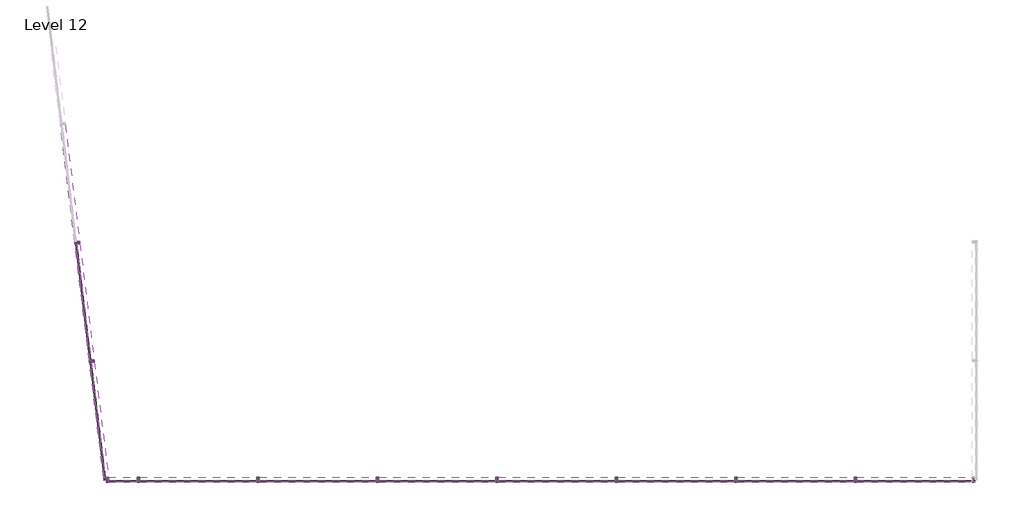
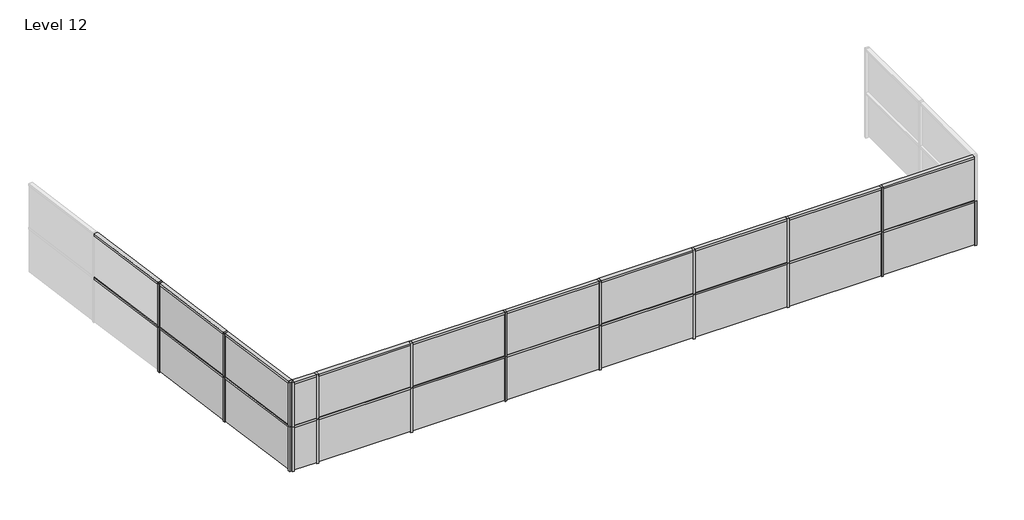
# One storey, part 1 of 2: 45 members, 20 plates.
"""IFC4 building model written with IfcOpenShell, lengths in millimetres."""

from ifc_helpers import new_model, si_unit, origin, place, context, project, spatial, transform, mapped, element, save
from components import member_daa7a266, member_82905deb, member_19d0a4ec, member_8cef0660, member_db480205, member_4491d118, member_0c11e56c, member_695b83e4, system_panel_glazed_37f15d2e, system_panel_glazed_3620f98e, system_panel_glazed_e46d4b42, system_panel_glazed_2a6c68b7, system_panel_glazed_07b088f8, system_panel_glazed_9d0e0944

model = new_model("IFC4")

# Units and contexts
model_context = context("Model", 3, world=origin())
ifc_project = project(units=[si_unit("LENGTHUNIT", "METRE", prefix="MILLI")], contexts=[model_context])

# Site, building, storey
site = spatial("IfcSite", under=ifc_project)
building = spatial("IfcBuilding", under=site)
storey = spatial("IfcBuildingStorey", under=building, Name="Level 12", Elevation=33528.0)

# Members
placement = place(None, origin())
member_shape = member_daa7a266(model_context)
element("IfcMember", 1, ObjectType="Rectangular Mullion : 2.5\" x 5\" rectangular", at=placement, inside=storey, context=model_context, shape_type="MappedRepresentation", body=[
    mapped(member_shape, transform((-8260.4765148, -6916.1096898, 36576.0), x_axis=(0.0, 0.0, 1.0), y_axis=(-0.9925461516413222, -0.12186934340514587, 0.0), z_axis=(0.12186934340514587, -0.9925461516413222, 0.0))),
])
element("IfcMember", 2, ObjectType="Rectangular Mullion : 2.5\" x 5\" rectangular", at=placement, inside=storey, context=model_context, shape_type="MappedRepresentation", body=[
    mapped(member_shape, transform((13839.0156363, -6979.1363705, 36576.0), x_axis=(0.0, 0.0, 1.0), y_axis=(0.0, -1.0, 0.0), z_axis=(1.0, 0.0, 0.0))),
])
member_2_shape = member_82905deb(model_context)
element("IfcMember", 3, ObjectType="Rectangular Mullion : 2.5\" x 5\" rectangular", at=placement, inside=storey, context=model_context, shape_type="MappedRepresentation", body=[
    mapped(member_2_shape, transform((-8624.1955702, -3953.8557, 36576.0), x_axis=(-0.1218693434051459, 0.9925461516413222, 0.0), y_axis=(-0.9925461516413222, -0.1218693434051459, 0.0), z_axis=(0.0, 0.0, 1.0))),
])
element("IfcMember", 4, ObjectType="Rectangular Mullion : 2.5\" x 5\" rectangular", at=placement, inside=storey, context=model_context, shape_type="MappedRepresentation", body=[
    mapped(member_2_shape, transform((-8995.6533289, -928.5750297, 36576.0), x_axis=(-0.1218693434051459, 0.9925461516413222, 0.0), y_axis=(-0.9925461516413222, -0.1218693434051459, 0.0), z_axis=(0.0, 0.0, 1.0))),
])
element("IfcMember", 5, ObjectType="Rectangular Mullion : 2.5\" x 5\" rectangular", at=placement, inside=storey, context=model_context, shape_type="MappedRepresentation", body=[
    mapped(member_2_shape, transform((10854.515636, -6979.1363705, 36576.0), x_axis=(-1.0, 0.0, 0.0), y_axis=(0.0, -1.0, 0.0), z_axis=(0.0, 0.0, 1.0))),
])
element("IfcMember", 6, ObjectType="Rectangular Mullion : 2.5\" x 5\" rectangular", at=placement, inside=storey, context=model_context, shape_type="MappedRepresentation", body=[
    mapped(member_2_shape, transform((7806.515636, -6979.1363705, 36576.0), x_axis=(-1.0, 0.0, 0.0), y_axis=(0.0, -1.0, 0.0), z_axis=(0.0, 0.0, 1.0))),
])
element("IfcMember", 7, ObjectType="Rectangular Mullion : 2.5\" x 5\" rectangular", at=placement, inside=storey, context=model_context, shape_type="MappedRepresentation", body=[
    mapped(member_2_shape, transform((4758.515636, -6979.1363705, 36576.0), x_axis=(-1.0, 0.0, 0.0), y_axis=(0.0, -1.0, 0.0), z_axis=(0.0, 0.0, 1.0))),
])
element("IfcMember", 8, ObjectType="Rectangular Mullion : 2.5\" x 5\" rectangular", at=placement, inside=storey, context=model_context, shape_type="MappedRepresentation", body=[
    mapped(member_2_shape, transform((1710.515636, -6979.1363705, 36576.0), x_axis=(-1.0, 0.0, 0.0), y_axis=(0.0, -1.0, 0.0), z_axis=(0.0, 0.0, 1.0))),
])
element("IfcMember", 9, ObjectType="Rectangular Mullion : 2.5\" x 5\" rectangular", at=placement, inside=storey, context=model_context, shape_type="MappedRepresentation", body=[
    mapped(member_2_shape, transform((-1337.484364, -6979.1363705, 36576.0), x_axis=(-1.0, 0.0, 0.0), y_axis=(0.0, -1.0, 0.0), z_axis=(0.0, 0.0, 1.0))),
])
element("IfcMember", 10, ObjectType="Rectangular Mullion : 2.5\" x 5\" rectangular", at=placement, inside=storey, context=model_context, shape_type="MappedRepresentation", body=[
    mapped(member_2_shape, transform((-4385.484364, -6979.1363705, 36576.0), x_axis=(-1.0, 0.0, 0.0), y_axis=(0.0, -1.0, 0.0), z_axis=(0.0, 0.0, 1.0))),
])
element("IfcMember", 11, ObjectType="Rectangular Mullion : 2.5\" x 5\" rectangular", at=placement, inside=storey, context=model_context, shape_type="MappedRepresentation", body=[
    mapped(member_2_shape, transform((-7433.484364, -6979.1363705, 36576.0), x_axis=(-1.0, 0.0, 0.0), y_axis=(0.0, -1.0, 0.0), z_axis=(0.0, 0.0, 1.0))),
])
member_3_shape = member_19d0a4ec(model_context)
element("IfcMember", 12, ObjectType="Rectangular Mullion : 2.5\" x 5\" rectangular", at=placement, inside=storey, context=model_context, shape_type="MappedRepresentation", body=[
    mapped(member_3_shape, transform((-8260.4765148, -6916.1096898, 35052.0), x_axis=(0.0, 0.0, 1.0), y_axis=(-0.9925461516413222, -0.12186934340514567, 0.0), z_axis=(0.12186934340514567, -0.9925461516413222, 0.0))),
])
element("IfcMember", 13, ObjectType="Rectangular Mullion : 2.5\" x 5\" rectangular", at=placement, inside=storey, context=model_context, shape_type="MappedRepresentation", body=[
    mapped(member_3_shape, transform((13839.0156363, -6979.1363705, 35052.0), x_axis=(0.0, 0.0, 1.0), y_axis=(0.0, -1.0, 0.0), z_axis=(1.0, 0.0, 0.0))),
])
member_4_shape = member_8cef0660(model_context)
element("IfcMember", 14, ObjectType="Rectangular Mullion : 2.5\" x 5\" rectangular", at=placement, inside=storey, context=model_context, shape_type="MappedRepresentation", body=[
    mapped(member_4_shape, transform((-8628.0649219, -3922.3423596, 35052.0), x_axis=(0.0, 0.0, 1.0), y_axis=(-0.9925461516413222, -0.12186934340514603, 0.0), z_axis=(0.12186934340514603, -0.9925461516413222, 0.0))),
])
element("IfcMember", 15, ObjectType="Rectangular Mullion : 2.5\" x 5\" rectangular", at=placement, inside=storey, context=model_context, shape_type="MappedRepresentation", body=[
    mapped(member_4_shape, transform((-8999.5226806, -897.0616894, 35052.0), x_axis=(0.0, 0.0, 1.0), y_axis=(-0.9925461516413222, -0.12186934340514596, 0.0), z_axis=(0.12186934340514596, -0.9925461516413222, 0.0))),
])
element("IfcMember", 16, ObjectType="Rectangular Mullion : 2.5\" x 5\" rectangular", at=placement, inside=storey, context=model_context, shape_type="MappedRepresentation", body=[
    mapped(member_4_shape, transform((10822.765636, -6979.1363705, 35052.0), x_axis=(0.0, 0.0, 1.0), y_axis=(0.0, -1.0, 0.0), z_axis=(1.0, 0.0, 0.0))),
])
element("IfcMember", 17, ObjectType="Rectangular Mullion : 2.5\" x 5\" rectangular", at=placement, inside=storey, context=model_context, shape_type="MappedRepresentation", body=[
    mapped(member_4_shape, transform((7774.765636, -6979.1363705, 35052.0), x_axis=(0.0, 0.0, 1.0), y_axis=(0.0, -1.0, 0.0), z_axis=(1.0, 0.0, 0.0))),
])
element("IfcMember", 18, ObjectType="Rectangular Mullion : 2.5\" x 5\" rectangular", at=placement, inside=storey, context=model_context, shape_type="MappedRepresentation", body=[
    mapped(member_4_shape, transform((4726.765636, -6979.1363705, 35052.0), x_axis=(0.0, 0.0, 1.0), y_axis=(0.0, -1.0, 0.0), z_axis=(1.0, 0.0, 0.0))),
])
element("IfcMember", 19, ObjectType="Rectangular Mullion : 2.5\" x 5\" rectangular", at=placement, inside=storey, context=model_context, shape_type="MappedRepresentation", body=[
    mapped(member_4_shape, transform((1678.765636, -6979.1363705, 35052.0), x_axis=(0.0, 0.0, 1.0), y_axis=(0.0, -1.0, 0.0), z_axis=(1.0, 0.0, 0.0))),
])
element("IfcMember", 20, ObjectType="Rectangular Mullion : 2.5\" x 5\" rectangular", at=placement, inside=storey, context=model_context, shape_type="MappedRepresentation", body=[
    mapped(member_4_shape, transform((-1369.234364, -6979.1363705, 35052.0), x_axis=(0.0, 0.0, 1.0), y_axis=(0.0, -1.0, 0.0), z_axis=(1.0, 0.0, 0.0))),
])
element("IfcMember", 21, ObjectType="Rectangular Mullion : 2.5\" x 5\" rectangular", at=placement, inside=storey, context=model_context, shape_type="MappedRepresentation", body=[
    mapped(member_4_shape, transform((-4417.234364, -6979.1363705, 35052.0), x_axis=(0.0, 0.0, 1.0), y_axis=(0.0, -1.0, 0.0), z_axis=(1.0, 0.0, 0.0))),
])
member_5_shape = member_db480205(model_context)
element("IfcMember", 22, ObjectType="Rectangular Mullion : 2.5\" x 5\" rectangular", at=placement, inside=storey, context=model_context, shape_type="MappedRepresentation", body=[
    mapped(member_5_shape, transform((-8628.0649219, -3922.3423596, 36576.0), x_axis=(0.0, 0.0, 1.0), y_axis=(-0.9925461516413222, -0.12186934340514599, 0.0), z_axis=(0.12186934340514599, -0.9925461516413222, 0.0))),
])
element("IfcMember", 23, ObjectType="Rectangular Mullion : 2.5\" x 5\" rectangular", at=placement, inside=storey, context=model_context, shape_type="MappedRepresentation", body=[
    mapped(member_5_shape, transform((-8999.5226806, -897.0616894, 36576.0), x_axis=(0.0, 0.0, 1.0), y_axis=(-0.9925461516413222, -0.12186934340514596, 0.0), z_axis=(0.12186934340514596, -0.9925461516413222, 0.0))),
])
element("IfcMember", 24, ObjectType="Rectangular Mullion : 2.5\" x 5\" rectangular", at=placement, inside=storey, context=model_context, shape_type="MappedRepresentation", body=[
    mapped(member_5_shape, transform((10822.765636, -6979.1363705, 36576.0), x_axis=(0.0, 0.0, 1.0), y_axis=(0.0, -1.0, 0.0), z_axis=(1.0, 0.0, 0.0))),
])
element("IfcMember", 25, ObjectType="Rectangular Mullion : 2.5\" x 5\" rectangular", at=placement, inside=storey, context=model_context, shape_type="MappedRepresentation", body=[
    mapped(member_5_shape, transform((7774.765636, -6979.1363705, 36576.0), x_axis=(0.0, 0.0, 1.0), y_axis=(0.0, -1.0, 0.0), z_axis=(1.0, 0.0, 0.0))),
])
element("IfcMember", 26, ObjectType="Rectangular Mullion : 2.5\" x 5\" rectangular", at=placement, inside=storey, context=model_context, shape_type="MappedRepresentation", body=[
    mapped(member_5_shape, transform((4726.765636, -6979.1363705, 36576.0), x_axis=(0.0, 0.0, 1.0), y_axis=(0.0, -1.0, 0.0), z_axis=(1.0, 0.0, 0.0))),
])
element("IfcMember", 27, ObjectType="Rectangular Mullion : 2.5\" x 5\" rectangular", at=placement, inside=storey, context=model_context, shape_type="MappedRepresentation", body=[
    mapped(member_5_shape, transform((1678.765636, -6979.1363705, 36576.0), x_axis=(0.0, 0.0, 1.0), y_axis=(0.0, -1.0, 0.0), z_axis=(1.0, 0.0, 0.0))),
])
element("IfcMember", 28, ObjectType="Rectangular Mullion : 2.5\" x 5\" rectangular", at=placement, inside=storey, context=model_context, shape_type="MappedRepresentation", body=[
    mapped(member_5_shape, transform((-1369.234364, -6979.1363705, 36576.0), x_axis=(0.0, 0.0, 1.0), y_axis=(0.0, -1.0, 0.0), z_axis=(1.0, 0.0, 0.0))),
])
element("IfcMember", 29, ObjectType="Rectangular Mullion : 2.5\" x 5\" rectangular", at=placement, inside=storey, context=model_context, shape_type="MappedRepresentation", body=[
    mapped(member_5_shape, transform((-4417.234364, -6979.1363705, 36576.0), x_axis=(0.0, 0.0, 1.0), y_axis=(0.0, -1.0, 0.0), z_axis=(1.0, 0.0, 0.0))),
])
element("IfcMember", 30, ObjectType="Rectangular Mullion : 2.5\" x 5\" rectangular", at=placement, inside=storey, context=model_context, shape_type="MappedRepresentation", body=[
    mapped(member_2_shape, transform((-8624.1955702, -3953.8557, 35052.0), x_axis=(-0.1218693434051459, 0.9925461516413222, 0.0), y_axis=(-0.9925461516413222, -0.1218693434051459, 0.0), z_axis=(0.0, 0.0, 1.0))),
])
element("IfcMember", 31, ObjectType="Rectangular Mullion : 2.5\" x 5\" rectangular", at=placement, inside=storey, context=model_context, shape_type="MappedRepresentation", body=[
    mapped(member_2_shape, transform((-8995.6533289, -928.5750297, 35052.0), x_axis=(-0.1218693434051459, 0.9925461516413222, 0.0), y_axis=(-0.9925461516413222, -0.1218693434051459, 0.0), z_axis=(0.0, 0.0, 1.0))),
])
element("IfcMember", 32, ObjectType="Rectangular Mullion : 2.5\" x 5\" rectangular", at=placement, inside=storey, context=model_context, shape_type="MappedRepresentation", body=[
    mapped(member_2_shape, transform((10854.515636, -6979.1363705, 35052.0), x_axis=(-1.0, 0.0, 0.0), y_axis=(0.0, -1.0, 0.0), z_axis=(0.0, 0.0, 1.0))),
])
element("IfcMember", 33, ObjectType="Rectangular Mullion : 2.5\" x 5\" rectangular", at=placement, inside=storey, context=model_context, shape_type="MappedRepresentation", body=[
    mapped(member_2_shape, transform((7806.515636, -6979.1363705, 35052.0), x_axis=(-1.0, 0.0, 0.0), y_axis=(0.0, -1.0, 0.0), z_axis=(0.0, 0.0, 1.0))),
])
element("IfcMember", 34, ObjectType="Rectangular Mullion : 2.5\" x 5\" rectangular", at=placement, inside=storey, context=model_context, shape_type="MappedRepresentation", body=[
    mapped(member_2_shape, transform((4758.515636, -6979.1363705, 35052.0), x_axis=(-1.0, 0.0, 0.0), y_axis=(0.0, -1.0, 0.0), z_axis=(0.0, 0.0, 1.0))),
])
element("IfcMember", 35, ObjectType="Rectangular Mullion : 2.5\" x 5\" rectangular", at=placement, inside=storey, context=model_context, shape_type="MappedRepresentation", body=[
    mapped(member_2_shape, transform((1710.515636, -6979.1363705, 35052.0), x_axis=(-1.0, 0.0, 0.0), y_axis=(0.0, -1.0, 0.0), z_axis=(0.0, 0.0, 1.0))),
])
element("IfcMember", 36, ObjectType="Rectangular Mullion : 2.5\" x 5\" rectangular", at=placement, inside=storey, context=model_context, shape_type="MappedRepresentation", body=[
    mapped(member_2_shape, transform((-1337.484364, -6979.1363705, 35052.0), x_axis=(-1.0, 0.0, 0.0), y_axis=(0.0, -1.0, 0.0), z_axis=(0.0, 0.0, 1.0))),
])
element("IfcMember", 37, ObjectType="Rectangular Mullion : 2.5\" x 5\" rectangular", at=placement, inside=storey, context=model_context, shape_type="MappedRepresentation", body=[
    mapped(member_2_shape, transform((-4385.484364, -6979.1363705, 35052.0), x_axis=(-1.0, 0.0, 0.0), y_axis=(0.0, -1.0, 0.0), z_axis=(0.0, 0.0, 1.0))),
])
element("IfcMember", 38, ObjectType="Rectangular Mullion : 2.5\" x 5\" rectangular", at=placement, inside=storey, context=model_context, shape_type="MappedRepresentation", body=[
    mapped(member_2_shape, transform((-7433.484364, -6979.1363705, 35052.0), x_axis=(-1.0, 0.0, 0.0), y_axis=(0.0, -1.0, 0.0), z_axis=(0.0, 0.0, 1.0))),
])
member_6_shape = member_4491d118(model_context)
element("IfcMember", 39, ObjectType="Rectangular Mullion : 2.5\" x 5\" rectangular", at=placement, inside=storey, context=model_context, shape_type="MappedRepresentation", body=[
    mapped(member_6_shape, transform((-8252.7378115, -6979.1363705, 36576.0), x_axis=(-1.0, 0.0, 0.0), y_axis=(0.0, -1.0, 0.0), z_axis=(0.0, 0.0, 1.0))),
])
element("IfcMember", 40, ObjectType="Rectangular Mullion : 2.5\" x 5\" rectangular", at=placement, inside=storey, context=model_context, shape_type="MappedRepresentation", body=[
    mapped(member_6_shape, transform((-8252.7378115, -6979.1363705, 33528.0), x_axis=(0.1218693434051459, -0.9925461516413222, 0.0), y_axis=(-0.9925461516413222, -0.1218693434051459, 0.0), z_axis=(0.0, 0.0, -1.0))),
])
element("IfcMember", 41, ObjectType="Rectangular Mullion : 2.5\" x 5\" rectangular", at=placement, inside=storey, context=model_context, shape_type="MappedRepresentation", body=[
    mapped(member_6_shape, transform((13902.5156363, -6979.1363705, 33528.0), x_axis=(1.0, 0.0, 0.0), y_axis=(0.0, -1.0, 0.0), z_axis=(0.0, 0.0, -1.0))),
])
element("IfcMember", 42, ObjectType="Rectangular Mullion : 2.5\" x 5\" rectangular", at=placement, inside=storey, context=model_context, shape_type="MappedRepresentation", body=[
    mapped(member_6_shape, transform((-8252.7378115, -6979.1363705, 35052.0), x_axis=(0.1218693434051459, -0.9925461516413222, 0.0), y_axis=(-0.9925461516413222, -0.1218693434051459, 0.0), z_axis=(0.0, 0.0, -1.0))),
])
element("IfcMember", 43, ObjectType="Rectangular Mullion : 2.5\" x 5\" rectangular", at=placement, inside=storey, context=model_context, shape_type="MappedRepresentation", body=[
    mapped(member_6_shape, transform((-8252.7378115, -6979.1363705, 35052.0), x_axis=(-1.0, 0.0, 0.0), y_axis=(0.0, -1.0, 0.0), z_axis=(0.0, 0.0, 1.0))),
])
member_7_shape = member_0c11e56c(model_context)
element("IfcMember", 44, ObjectType="Rectangular Mullion : 2.5\" x 5\" rectangular", at=placement, inside=storey, context=model_context, shape_type="MappedRepresentation", body=[
    mapped(member_7_shape, transform((-7465.234364, -6979.1363705, 35052.0), x_axis=(0.0, 0.0, 1.0), y_axis=(0.0, -1.0, 0.0), z_axis=(1.0, 0.0, 0.0))),
])
member_8_shape = member_695b83e4(model_context)
element("IfcMember", 45, ObjectType="Rectangular Mullion : 2.5\" x 5\" rectangular", at=placement, inside=storey, context=model_context, shape_type="MappedRepresentation", body=[
    mapped(member_8_shape, transform((-7465.234364, -6979.1363705, 36576.0), x_axis=(0.0, 0.0, 1.0), y_axis=(0.0, -1.0, 0.0), z_axis=(1.0, 0.0, 0.0))),
])

# Plates
system_panel_glazed_shape = system_panel_glazed_37f15d2e(model_context)
element("IfcPlate", 46, ObjectType="System Panel : Glazed", at=placement, inside=storey, context=model_context, shape_type="MappedRepresentation", body=[
    mapped(system_panel_glazed_shape, transform((-8440.4013667, -5450.739365, 35083.75), x_axis=(-0.1218693434051459, 0.9925461516413222, 0.0), y_axis=(-0.9925461516413222, -0.1218693434051459, 0.0), z_axis=(0.0, 0.0, 1.0))),
])
element("IfcPlate", 47, ObjectType="System Panel : Glazed", at=placement, inside=storey, context=model_context, shape_type="MappedRepresentation", body=[
    mapped(system_panel_glazed_shape, transform((12362.6406361, -6979.1363705, 35083.75), x_axis=(-1.0, 0.0, 0.0), y_axis=(0.0, -1.0, 0.0), z_axis=(0.0, 0.0, 1.0))),
])
system_panel_glazed_2_shape = system_panel_glazed_3620f98e(model_context)
element("IfcPlate", 48, ObjectType="System Panel : Glazed", at=placement, inside=storey, context=model_context, shape_type="MappedRepresentation", body=[
    mapped(system_panel_glazed_2_shape, transform((-8809.9244496, -2441.2153649, 35083.75), x_axis=(-0.1218693434051459, 0.9925461516413222, 0.0), y_axis=(-0.9925461516413222, -0.1218693434051459, 0.0), z_axis=(0.0, 0.0, 1.0))),
])
element("IfcPlate", 49, ObjectType="System Panel : Glazed", at=placement, inside=storey, context=model_context, shape_type="MappedRepresentation", body=[
    mapped(system_panel_glazed_2_shape, transform((9330.515636, -6979.1363705, 35083.75), x_axis=(-1.0, 0.0, 0.0), y_axis=(0.0, -1.0, 0.0), z_axis=(0.0, 0.0, 1.0))),
])
element("IfcPlate", 50, ObjectType="System Panel : Glazed", at=placement, inside=storey, context=model_context, shape_type="MappedRepresentation", body=[
    mapped(system_panel_glazed_2_shape, transform((6282.515636, -6979.1363705, 35083.75), x_axis=(-1.0, 0.0, 0.0), y_axis=(0.0, -1.0, 0.0), z_axis=(0.0, 0.0, 1.0))),
])
element("IfcPlate", 51, ObjectType="System Panel : Glazed", at=placement, inside=storey, context=model_context, shape_type="MappedRepresentation", body=[
    mapped(system_panel_glazed_2_shape, transform((3234.515636, -6979.1363705, 35083.75), x_axis=(-1.0, 0.0, 0.0), y_axis=(0.0, -1.0, 0.0), z_axis=(0.0, 0.0, 1.0))),
])
element("IfcPlate", 52, ObjectType="System Panel : Glazed", at=placement, inside=storey, context=model_context, shape_type="MappedRepresentation", body=[
    mapped(system_panel_glazed_2_shape, transform((186.515636, -6979.1363705, 35083.75), x_axis=(-1.0, 0.0, 0.0), y_axis=(0.0, -1.0, 0.0), z_axis=(0.0, 0.0, 1.0))),
])
element("IfcPlate", 53, ObjectType="System Panel : Glazed", at=placement, inside=storey, context=model_context, shape_type="MappedRepresentation", body=[
    mapped(system_panel_glazed_2_shape, transform((-2861.484364, -6979.1363705, 35083.75), x_axis=(-1.0, 0.0, 0.0), y_axis=(0.0, -1.0, 0.0), z_axis=(0.0, 0.0, 1.0))),
])
element("IfcPlate", 54, ObjectType="System Panel : Glazed", at=placement, inside=storey, context=model_context, shape_type="MappedRepresentation", body=[
    mapped(system_panel_glazed_2_shape, transform((-5909.484364, -6979.1363705, 35083.75), x_axis=(-1.0, 0.0, 0.0), y_axis=(0.0, -1.0, 0.0), z_axis=(0.0, 0.0, 1.0))),
])
system_panel_glazed_3_shape = system_panel_glazed_e46d4b42(model_context)
element("IfcPlate", 55, ObjectType="System Panel : Glazed", at=placement, inside=storey, context=model_context, shape_type="MappedRepresentation", body=[
    mapped(system_panel_glazed_3_shape, transform((-8440.4013667, -5450.739365, 33559.75), x_axis=(-0.1218693434051459, 0.9925461516413222, 0.0), y_axis=(-0.9925461516413222, -0.1218693434051459, 0.0), z_axis=(0.0, 0.0, 1.0))),
])
element("IfcPlate", 56, ObjectType="System Panel : Glazed", at=placement, inside=storey, context=model_context, shape_type="MappedRepresentation", body=[
    mapped(system_panel_glazed_3_shape, transform((12362.6406361, -6979.1363705, 33559.75), x_axis=(-1.0, 0.0, 0.0), y_axis=(0.0, -1.0, 0.0), z_axis=(0.0, 0.0, 1.0))),
])
system_panel_glazed_4_shape = system_panel_glazed_2a6c68b7(model_context)
element("IfcPlate", 57, ObjectType="System Panel : Glazed", at=placement, inside=storey, context=model_context, shape_type="MappedRepresentation", body=[
    mapped(system_panel_glazed_4_shape, transform((-8809.9244496, -2441.2153649, 33559.75), x_axis=(-0.1218693434051459, 0.9925461516413222, 0.0), y_axis=(-0.9925461516413222, -0.1218693434051459, 0.0), z_axis=(0.0, 0.0, 1.0))),
])
element("IfcPlate", 58, ObjectType="System Panel : Glazed", at=placement, inside=storey, context=model_context, shape_type="MappedRepresentation", body=[
    mapped(system_panel_glazed_4_shape, transform((9330.515636, -6979.1363705, 33559.75), x_axis=(-1.0, 0.0, 0.0), y_axis=(0.0, -1.0, 0.0), z_axis=(0.0, 0.0, 1.0))),
])
element("IfcPlate", 59, ObjectType="System Panel : Glazed", at=placement, inside=storey, context=model_context, shape_type="MappedRepresentation", body=[
    mapped(system_panel_glazed_4_shape, transform((6282.515636, -6979.1363705, 33559.75), x_axis=(-1.0, 0.0, 0.0), y_axis=(0.0, -1.0, 0.0), z_axis=(0.0, 0.0, 1.0))),
])
element("IfcPlate", 60, ObjectType="System Panel : Glazed", at=placement, inside=storey, context=model_context, shape_type="MappedRepresentation", body=[
    mapped(system_panel_glazed_4_shape, transform((3234.515636, -6979.1363705, 33559.75), x_axis=(-1.0, 0.0, 0.0), y_axis=(0.0, -1.0, 0.0), z_axis=(0.0, 0.0, 1.0))),
])
element("IfcPlate", 61, ObjectType="System Panel : Glazed", at=placement, inside=storey, context=model_context, shape_type="MappedRepresentation", body=[
    mapped(system_panel_glazed_4_shape, transform((186.515636, -6979.1363705, 33559.75), x_axis=(-1.0, 0.0, 0.0), y_axis=(0.0, -1.0, 0.0), z_axis=(0.0, 0.0, 1.0))),
])
element("IfcPlate", 62, ObjectType="System Panel : Glazed", at=placement, inside=storey, context=model_context, shape_type="MappedRepresentation", body=[
    mapped(system_panel_glazed_4_shape, transform((-2861.484364, -6979.1363705, 33559.75), x_axis=(-1.0, 0.0, 0.0), y_axis=(0.0, -1.0, 0.0), z_axis=(0.0, 0.0, 1.0))),
])
element("IfcPlate", 63, ObjectType="System Panel : Glazed", at=placement, inside=storey, context=model_context, shape_type="MappedRepresentation", body=[
    mapped(system_panel_glazed_4_shape, transform((-5909.484364, -6979.1363705, 33559.75), x_axis=(-1.0, 0.0, 0.0), y_axis=(0.0, -1.0, 0.0), z_axis=(0.0, 0.0, 1.0))),
])
system_panel_glazed_5_shape = system_panel_glazed_07b088f8(model_context)
element("IfcPlate", 64, ObjectType="System Panel : Glazed", at=placement, inside=storey, context=model_context, shape_type="MappedRepresentation", body=[
    mapped(system_panel_glazed_5_shape, transform((-7827.2360878, -6979.1363705, 35083.75), x_axis=(-1.0, 0.0, 0.0), y_axis=(0.0, -1.0, 0.0), z_axis=(0.0, 0.0, 1.0))),
])
system_panel_glazed_6_shape = system_panel_glazed_9d0e0944(model_context)
element("IfcPlate", 65, ObjectType="System Panel : Glazed", at=placement, inside=storey, context=model_context, shape_type="MappedRepresentation", body=[
    mapped(system_panel_glazed_6_shape, transform((-7827.2360878, -6979.1363705, 33559.75), x_axis=(-1.0, 0.0, 0.0), y_axis=(0.0, -1.0, 0.0), z_axis=(0.0, 0.0, 1.0))),
])

save(model, "model.ifc")

# Revit data of these elements
# Type "Rectangular Mullion : 2.5\" x 5\" rectangular"
#   built-in parameter 1007304 = 0.416667 (stored number, unit not read)
#   built-in parameter 1007301 = 0.104167 (stored number, unit not read)
#   built-in parameter 1007300 = 0.104167 (stored number, unit not read)
# Type "System Panel : Glazed"
#   Construction Type Id = "GSP4R"
#   Analytic Construction = "1/8 in Pilkington single glazing"
#   Visual Light Transmittance = 0.9
#   Solar Heat Gain Coefficient = 0.86
#   Heat Transfer Coefficient (U) = 1.18115 BTU/(h·ft²·°F)
#   Define Thermal Properties by = 1
# Elements 1, 2, 3, 4, 5, 6, 7, 8, 9, 10, 11, 12, 13, 14, 15, 16, 17, 18, 19, 20, 21, 22, 23, 24, 25, 26, 27, 28, 29, 30, 31, 32, 33, 34, 35, 36, 37, 38, 39, 40, 41, 42, 43, 44, 45 (IfcMember, "Rectangular Mullion : 2.5\" x 5\" rectangular")
#   Phase Created = New Construction
#   Materials on its faces: "Aluminum"
# Elements 46, 47, 48, 49, 50, 51, 52, 53, 54, 55, 56, 57, 58, 59, 60, 61, 62, 63, 64, 65 (IfcPlate, "System Panel : Glazed")
#   Phase Created = New Construction
#   Materials on its faces: "Glass"
# Materials
#   "Aluminum": class "Metal", colour RGB 247 247 247, transparency 0, Description = "Aluminum 6061", Cost = 0
#   "Glass": class "Glass", colour RGB 0 128 192, transparency 0.75, Description = "Soda Lime Glass", Cost = 0
